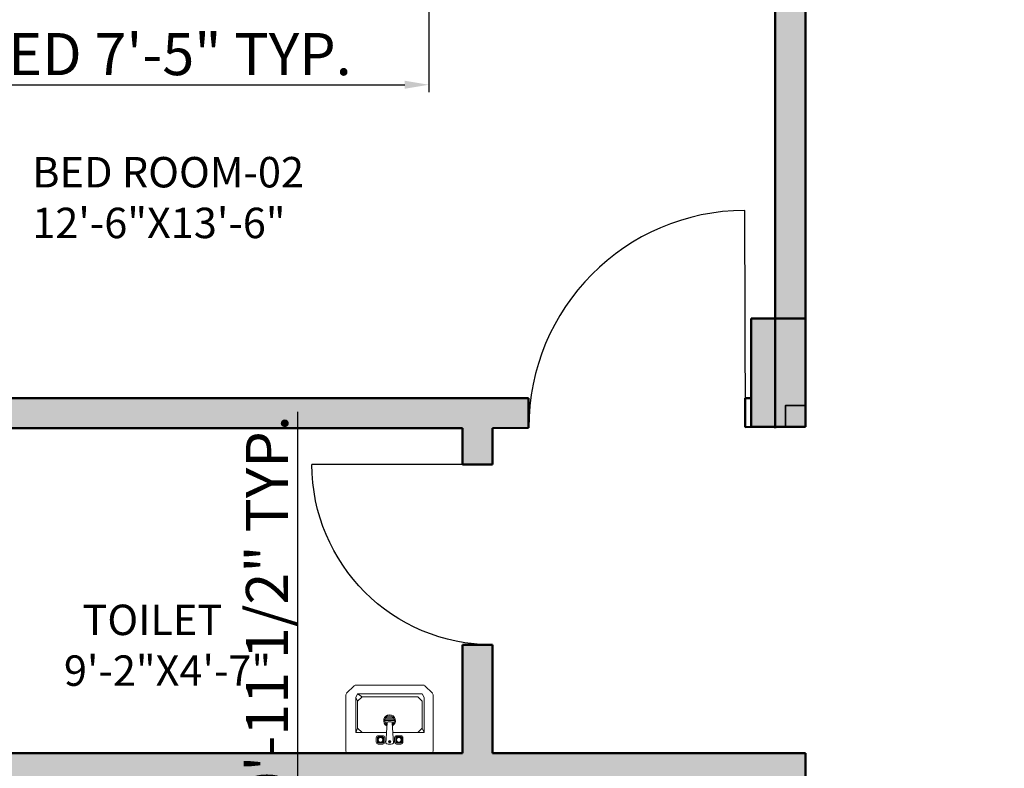
# Model space of a CAD drawing. Units: inches. Extents: x -7 to 1228, y -146 to 1091.
# Tile 10 of 88: x 105 to 269, y 276 to 401. Entities that reach past the tile are written whole.
import ezdxf

# ---------------------------------------------------------------- set-up
doc = ezdxf.new("R2010")
doc.units = ezdxf.units.IN
for name, color, linetype, lineweight in [('A-ANNO-DIMS', 2, 'Continuous', 18), ('A-AREA-IDEN', 7, 'Continuous', 18), ('A-COLS', 6, 'Continuous', 35), ('A-DOOR', 4, 'Continuous', 25), ('A-FURN', 8, 'Continuous', 18), ('A-WALL', 7, 'Continuous', 50), ('A-WALL-PATT', 251, 'Continuous', 13)]:
    doc.layers.add(name, color=color, linetype=linetype, lineweight=lineweight)
doc.styles.get("Standard").update_dxf_attribs({"font": 'arial.ttf'})
doc.dimstyles.new('ISO-25', dxfattribs={"dimtxt": 7, "dimasz": 4, "dimexe": 1.25, "dimexo": 0.625, "dimtad": 1, "dimdec": 1, "dimlunit": 3, "dimtxsty": 'Standard', "dimcen": 2.5, "dimadec": 0, "dimazin": 0, "dimtfac": 1, "dimtdec": 1, "dimtmove": 1, "dimatfit": 3, "dimfxl": 1, "dimarcsym": 0})

# ---------------------------------------------------------------- blocks, each defined once
blk = doc.blocks.new('A$C4CB854FF')
for p, q in [((0, 0.3675), (0, 0.0552)), ((0.4725, 0.38), (0.0125, 0.38)), ((0.1787, 0.329), (0.2034, 0.329)), ((0.2337, 0.329), (0.2502, 0.329)), ((0.3052, 0.329), (0.2804, 0.329)), ((0.485, 0.0552), (0.485, 0.3675)), ((0.1677, 0.2932), (0.1677, 0.318)), ((0.1745, 0.2919), (0.1745, 0.3194)), ((0.1773, 0.3221), (0.2048, 0.3221)), ((0.2048, 0.2891), (0.1773, 0.2891)), ((0.2034, 0.2822), (0.1787, 0.2822)), ((0.2075, 0.3194), (0.2075, 0.2919)), ((0.2144, 0.318), (0.2144, 0.2932)), ((0.2279, 0.2104), (0.2213, 0.3235)), ((0.2625, 0.3235), (0.256, 0.2104)), ((0.2694, 0.318), (0.2694, 0.2932)), ((0.2763, 0.3194), (0.2763, 0.2919)), ((0.3065, 0.3221), (0.279, 0.3221)), ((0.279, 0.2891), (0.3065, 0.2891)), ((0.2804, 0.2822), (0.3052, 0.2822)), ((0.3093, 0.2919), (0.3093, 0.3194)), ((0.3162, 0.2932), (0.3162, 0.318)), ((0.05, 0.265), (0.2247, 0.265)), ((0.06, 0.24), (0.05, 0.265)), ((0.05, 0.07), (0.05, 0.265)), ((0.085, 0.265), (0.06, 0.24)), ((0.06, 0.24), (0.06, 0.09)), ((0.2591, 0.265), (0.43, 0.265)), ((0.395, 0.265), (0.42, 0.24)), ((0.42, 0.24), (0.43, 0.265)), ((0.42, 0.24), (0.42, 0.09)), ((0.43, 0.07), (0.43, 0.265)), ((0.2152, 0.1984), (0.2694, 0.1984)), ((0.2297, 0.2066), (0.2165, 0.2066)), ((0.2681, 0.1901), (0.2165, 0.1901)), ((0.2272, 0.2149), (0.2208, 0.2149)), ((0.2638, 0.1819), (0.2208, 0.1819)), ((0.2533, 0.1736), (0.2313, 0.1736)), ((0.2505, 0.2052), (0.2334, 0.2052)), ((0.2681, 0.2066), (0.2541, 0.2066)), ((0.2638, 0.2149), (0.2566, 0.2149)), ((0.05, 0.07), (0.06, 0.05)), ((0.06, 0.09), (0.085, 0.065)), ((0.085, 0.065), (0.395, 0.065)), ((0.42, 0.09), (0.395, 0.065)), ((0.395, 0.065), (0.42, 0.05)), ((0.42, 0.09), (0.43, 0.07)), ((0.43, 0.07), (0.42, 0.05)), ((0.0037, 0.0463), (0.0463, 0.0037)), ((0.42, 0.05), (0.06, 0.05)), ((0.4387, 0.0037), (0.4813, 0.0463)), ((0.0552, 0), (0.4298, 0))]:
    blk.add_line(p, q)
for centre, radius in [((0.191, 0.3056), 0.0165), ((0.191, 0.3056), 0.0127), ((0.2419, 0.3152), 0.00688), ((0.2419, 0.3152), 0.00344), ((0.2928, 0.3056), 0.0165), ((0.2928, 0.3056), 0.0127)]:
    blk.add_circle(centre, radius)
for centre, radius, start, end in [((0.0125, 0.3675), 0.0125, 90, 180), ((0.1787, 0.318), 0.011, 90, 180), ((0.2034, 0.318), 0.011, 0, 90), ((0.2329, 0.314), 0.015, 87.1975, 140.7274), ((0.2509, 0.314), 0.015, 39.2726, 92.8025), ((0.2804, 0.318), 0.011, 90, 180), ((0.3052, 0.318), 0.011, 0, 90), ((0.4725, 0.3675), 0.0125, 0, 90), ((0.1787, 0.2932), 0.011, 180, 270), ((0.1773, 0.3194), 0.00275, 90, 180), ((0.1773, 0.2919), 0.00275, 180, 270), ((0.2034, 0.2932), 0.011, 270, 0), ((0.2048, 0.3194), 0.00275, 360, 90), ((0.2048, 0.2919), 0.00275, 270, 0), ((0.2804, 0.2932), 0.011, 180, 270), ((0.279, 0.3194), 0.00275, 90, 180), ((0.279, 0.2919), 0.00275, 180, 270), ((0.3052, 0.2932), 0.011, 270, 360), ((0.3065, 0.3194), 0.00275, 360, 90), ((0.3065, 0.2919), 0.00275, 270, 0), ((0.2423, 0.1984), 0.033, 118.6883, 62.8686), ((0.2423, 0.1984), 0.0271, 124.7758, 57.2247), ((0.2334, 0.2107), 0.0055, 183.3274, 270), ((0.2505, 0.2107), 0.0055, 270, 356.6726), ((0.0125, 0.0552), 0.0125, 180, 225), ((0.4725, 0.0552), 0.0125, 315, 0), ((0.0552, 0.0125), 0.0125, 225, 270), ((0.4298, 0.0125), 0.0125, 270, 315)]:
    blk.add_arc(centre, radius, start, end)
blk = doc.blocks.new('DOOR-750')
blk.add_line((30, 30), (30, 0))
blk.add_arc((30, 30), 30, 180, 270)
blk = doc.blocks.new('DOOR-900')
blk.add_line((36, 0), (36, 36))
blk.add_arc((36, 0), 36, 90, 180)
blk = doc.blocks.new('*D24')
at = {"layer": 'A-ANNO-DIMS', "color": 0, "lineweight": -2, "transparency": 16777216}
for p, q in [((84.44, 402.8), (84.44, 388.82)), ((173.43, 402.8), (173.43, 388.82)), ((88.44, 390.07), (169.43, 390.07))]:
    blk.add_line(p, q, dxfattribs=at)
at = {"layer": 'A-ANNO-DIMS', "color": 0, "transparency": 16777216}
for points in [[(88.44, 390.74), (88.44, 389.41), (84.44, 390.07)], [(169.43, 390.74), (169.43, 389.41), (173.43, 390.07)]]:
    blk.add_solid(points, dxfattribs=at)
at = {"layer": 'Defpoints', "color": 0, "transparency": 16777216}
for p in [(84.44, 403.42), (173.43, 403.42), (173.43, 390.07)]:
    blk.add_point(p, dxfattribs=at)
at = {"layer": 'A-ANNO-DIMS', "color": 0, "transparency": 16777216, "insert": (128.93, 394.26), "char_height": 7, "attachment_point": 5}
blk.add_mtext('BED 7\'-5" TYP.', dxfattribs=at)
blk = doc.blocks.new('*D32')
at = {"layer": 'A-ANNO-DIMS', "color": 0, "lineweight": -2, "transparency": 16777216}
for p, q in [((159.65, 262.03), (159.65, 259.24)), ((174.13, 262.03), (174.13, 259.24)), ((170.13, 260.49), (163.65, 260.49)), ((166.89, 260.49), (170.8, 247.44)), ((170.8, 247.44), (294.04, 247.44))]:
    blk.add_line(p, q, dxfattribs=at)
at = {"layer": 'A-ANNO-DIMS', "color": 0, "transparency": 16777216}
for points in [[(163.65, 261.15), (163.65, 259.82), (159.65, 260.49)], [(170.13, 261.15), (170.13, 259.82), (174.13, 260.49)]]:
    blk.add_solid(points, dxfattribs=at)
at = {"layer": 'Defpoints', "color": 0, "transparency": 16777216}
for p in [(159.65, 262.66), (174.13, 262.66), (159.65, 260.49)]:
    blk.add_point(p, dxfattribs=at)
at = {"layer": 'A-ANNO-DIMS', "color": 0, "transparency": 16777216, "insert": (232.42, 251.68), "char_height": 7, "attachment_point": 5}
blk.add_mtext('SINK / BASIN 1\'-2 1/2" TYP.', dxfattribs=at)
blk = doc.blocks.new('*D33')
at = {"layer": 'A-ANNO-DIMS', "color": 0, "lineweight": -2, "transparency": 16777216}
for p, q in [((151.67, 270.07), (151.67, 335.74)), ((159.03, 274), (156.23, 274)), ((157.48, 268.33), (151.67, 270.07)), ((157.48, 266.66), (157.48, 270)), ((159.03, 262.66), (156.23, 262.66))]:
    blk.add_line(p, q, dxfattribs=at)
at = {"layer": 'A-ANNO-DIMS', "color": 0, "transparency": 16777216}
for points in [[(156.81, 270), (158.15, 270), (157.48, 274)], [(156.81, 266.66), (158.15, 266.66), (157.48, 262.66)]]:
    blk.add_solid(points, dxfattribs=at)
at = {"layer": 'Defpoints', "color": 0, "transparency": 16777216}
for p in [(157.48, 274), (159.65, 274), (159.65, 262.66)]:
    blk.add_point(p, dxfattribs=at)
at = {"layer": 'A-ANNO-DIMS', "color": 0, "transparency": 16777216, "insert": (147.43, 302.9), "char_height": 7, "attachment_point": 5, "rotation": 90}
blk.add_mtext('0\'-11 1/2" TYP.', dxfattribs=at)

msp = doc.modelspace()

# ---------------------------------------------------------------- hatches: boundary and pattern name
at = {"layer": 'A-COLS'}
h = msp.add_hatch(color=256, dxfattribs=at)
h.dxf.hatch_style = 1
h.paths.add_polyline_path([(236, 351.24), (227, 351.24), (227, 333.24), (232.71, 333.24), (232.71, 336.78), (236, 336.78)])
h = msp.add_hatch(color=256, dxfattribs=at)
h.dxf.hatch_style = 1
h.paths.add_polyline_path([(232.71, 336.78), (232.71, 333.24), (236, 333.24), (236, 336.78)])
at = {"layer": 'A-WALL-PATT'}
h = msp.add_hatch(color=256, dxfattribs=at)
h.dxf.hatch_style = 1
h.paths.add_polyline_path([(69, 568), (60, 568), (60, 493), (63.29, 493), (69, 493)])
h.paths.add_polyline_path([(69, 662.41), (60, 662.41), (60, 586), (69, 586)], flags=17)
h.paths.add_polyline_path([(69, 723), (184, 723), (184, 734), (179, 734), (179, 728), (69, 728), (69, 741.62), (60, 741.62), (60, 698.41), (69, 698.41)], flags=17)
h.paths.add_polyline_path([(69, 782), (231, 782), (231, 728), (231, 723), (231, 586), (236, 586), (236, 787), (69, 787), (69, 800.13), (60, 800.13), (60, 765.62), (69, 765.62)])
h.paths.add_polyline_path([(184, 842), (189, 842), (189, 848), (173, 848), (173, 842), (179, 842), (179, 787), (184, 787)])
h.paths.add_polyline_path([(118.22, 69), (69, 69), (69, 60), (118.22, 60)])
h.paths.add_polyline_path([(227, 69), (154.22, 69), (154.22, 60), (227, 60)])
h.paths.add_polyline_path([(236, 60), (232.71, 60), (227, 60), (227, 36), (236, 36)])
h.paths.add_polyline_path([(389, 60), (380, 60), (380, 36), (389, 36)])
h.paths.add_polyline_path([(384, 181), (380, 181), (380, 115), (380, 78), (384, 78)])
h.paths.add_polyline_path([(380, 115), (334.55, 115), (334.55, 109), (380, 109)])
h.paths.add_polyline_path([(274.55, 115), (236, 115), (236, 201), (232.71, 201), (231, 201), (231, 78), (236, 78), (236, 109), (274.55, 109)])
h.paths.add_polyline_path([(69, 123), (60, 123), (60, 78), (69, 78)])
h.paths.add_polyline_path([(69, 201), (60, 201), (60, 159), (69, 159)])
h.paths.add_polyline_path([(143, 219), (69, 219), (69, 213), (143, 213)], flags=17)
h.paths.add_polyline_path([(189, 219), (184, 219), (184, 274), (231, 274), (231, 219), (236, 219), (236, 279), (184, 279), (184, 297), (179, 297), (179, 279), (69, 279), (69, 290.91), (60, 290.91), (60, 262.18), (69, 262.18), (69, 274), (179, 274), (179, 219), (173, 219), (173, 213), (189, 213)])
h.paths.add_polyline_path([(69, 238.18), (60, 238.18), (60, 219), (69, 219)], flags=17)
h.paths.add_polyline_path([(69, 333), (60, 333), (60, 314.91), (69, 314.91), (69, 316.96)])
h.paths.add_polyline_path([(190, 338), (184, 338), (69, 338), (69, 333), (179, 333), (179, 327), (184, 327), (184, 333.02), (190, 333.05)])
h.paths.add_polyline_path([(69, 386.81), (60, 386.81), (60, 351), (69, 351)])
h.paths.add_polyline_path([(69, 475), (60, 475), (60, 422.81), (69, 422.81)])
h.paths.add_polyline_path([(236, 475), (231, 475), (231, 351.24), (236, 351.24)])
h.paths.add_polyline_path([(384, 475), (380, 475), (380, 362), (384, 362)])
h.paths.add_polyline_path([(547, 307), (439, 307), (439, 356), (445, 356), (445, 362), (433, 362), (433, 307), (380, 307), (380, 244), (380, 241), (384, 241), (384, 301), (433, 301), (433, 277), (439, 277), (439, 301), (547, 301)])
h.paths.add_polyline_path([(547, 241), (439, 241), (439, 247), (433, 247), (433, 235), (547, 235)])
h.paths.add_polyline_path([(450, 69), (440.29, 69), (424.89, 69), (389, 69), (389, 60), (450, 60)])
h.paths.add_polyline_path([(547, 69), (486, 69), (486, 60), (547, 60)])
h.paths.add_polyline_path([(556, 148.27), (547, 148.27), (547, 78), (556, 78)])
h.paths.add_polyline_path([(556, 223), (547, 223), (547, 195), (547, 184.27), (556, 184.27)])
h.paths.add_polyline_path([(556, 311.19), (547, 311.19), (547, 273.08), (556, 273.08)])
h.paths.add_polyline_path([(556, 344), (552.71, 344), (547, 344), (547, 335.19), (556, 335.19)])
h.paths.add_polyline_path([(556, 249.08), (547, 249.08), (547, 241), (556, 241)])
h.paths.add_polyline_path([(547, 362), (475, 362), (475, 356), (547, 356)], flags=0)
h.paths.add_polyline_path([(556, 399.62), (547, 399.62), (547, 362), (556, 362)])
h.paths.add_polyline_path([(556, 475), (547, 475), (547, 435.62), (556, 435.62)])
h.paths.add_polyline_path([(547, 493), (389, 493), (389, 487), (547, 487)])
h.paths.add_polyline_path([(380, 493), (278, 493), (278, 487), (380, 487)])
h.paths.add_polyline_path([(227, 493), (69, 493), (69, 487), (227, 487)])
h.paths.add_polyline_path([(643, 122.44), (634, 122.44), (634, 78), (643, 78)])
h.paths.add_polyline_path([(702.5, 69), (692.79, 69), (677.39, 69), (643, 69), (643, 60), (702.5, 60)])
h.paths.add_polyline_path([(798, 69), (738.5, 69), (738.5, 60), (798, 60)])
h.paths.add_polyline_path([(807, 60), (803.71, 60), (798, 60), (798, 36), (807, 36)])
h.paths.add_polyline_path([(807, 109), (846.75, 109), (846.75, 115), (807, 115), (807, 159), (802, 159), (802, 78), (807, 78)])
h.paths.add_polyline_path([(807, 201), (802, 201), (802, 195), (807, 195)])
h.paths.add_polyline_path([(643, 201), (634, 201), (634, 158.44), (643, 158.44)])
h.paths.add_polyline_path([(756, 225), (751, 225), (751, 219), (643, 219), (643, 213), (756, 213)])
h.paths.add_polyline_path([(643, 240.85), (634, 240.85), (634, 219), (643, 219)])
h.paths.add_polyline_path([(643, 274), (643, 288.63), (634, 288.63), (634, 264.85), (643, 264.85)])
h.paths.add_polyline_path([(802, 279), (756, 279), (756, 297), (751, 297), (751, 279), (643, 279), (643, 274), (751, 274), (751, 255), (756, 255), (756, 274), (802, 274)])
h.paths.add_polyline_path([(807, 333), (803.71, 333), (802, 333), (802, 279), (802, 274), (802, 219), (807, 219)])
h.paths.add_polyline_path([(956, 182), (951, 182), (951, 115), (906.75, 115), (906.75, 109), (951, 109), (951, 78), (956, 78)])
h.paths.add_polyline_path([(960, 60), (951, 60), (951, 36), (960, 36)])
h.paths.add_polyline_path([(1021, 69), (1005.78, 69), (960, 69), (960, 60), (1021, 60)])
h.paths.add_polyline_path([(956, 224), (951, 224), (951, 218), (956, 218)])
h.paths.add_polyline_path([(956, 302), (1004, 302), (1004, 278), (1010, 278), (1010, 302), (1118, 302), (1118, 290.81), (1127, 290.81), (1127, 326.97), (1118, 326.97), (1118, 320.97), (1118, 307), (1010, 307), (1010, 356), (1016, 356), (1016, 362), (1004, 362), (1004, 307), (951, 307), (951, 244), (951, 242), (954.29, 242), (956, 242)])
h.paths.add_polyline_path([(643, 333), (634, 333), (634, 312.63), (643, 312.63), (643, 316.96)])
h.paths.add_polyline_path([(756, 338), (643, 338), (643, 333), (751, 333), (751, 327), (756, 327)])
h.paths.add_polyline_path([(643, 388), (634, 388), (634, 351), (643, 351)])
h.paths.add_polyline_path([(807, 357), (802, 357), (802, 351), (807, 351)])
h.paths.add_polyline_path([(807, 475), (802, 475), (802, 393), (807, 393)])
h.paths.add_polyline_path([(643, 475), (634, 475), (634, 424), (643, 424)])
h.paths.add_polyline_path([(798, 493), (643, 493), (643, 487), (798, 487)])
h.paths.add_polyline_path([(634, 493), (556, 493), (556, 487), (634, 487)])
h.paths.add_polyline_path([(813, 493), (807, 493), (807, 487), (813, 487)])
h.paths.add_polyline_path([(951, 493), (849, 493), (849, 487), (951, 487)])
h.paths.add_polyline_path([(956, 484), (951, 484), (951, 374), (956, 374)])
h.paths.add_polyline_path([(1109, 493), (969, 493), (969, 487), (1109, 487)])
h.paths.add_polyline_path([(1127, 484), (1118, 484), (1118, 450.64), (1127, 450.64)])
h.paths.add_polyline_path([(1127, 414.64), (1118, 414.64), (1118, 365), (1127, 365)])
h.paths.add_polyline_path([(1109, 362), (1046, 362), (1046, 356), (1109, 356)], flags=17)
h.paths.add_polyline_path([(1127, 356), (1123.45, 356), (1118, 356), (1118, 350.97), (1127, 350.97)], flags=0)
h.paths.add_polyline_path([(1127, 266.81), (1118, 266.81), (1118, 262.36), (1118, 242), (1127, 242)], flags=17)
h.paths.add_polyline_path([(1118, 242), (1010, 242), (1010, 248), (1004, 248), (1004, 237), (1118, 237)])
h.paths.add_polyline_path([(1127, 224), (1118, 224), (1118, 170), (1127, 170)])
h.paths.add_polyline_path([(1127, 134), (1118, 134), (1118, 78), (1127, 78)])
h.paths.add_polyline_path([(1118, 69), (1057, 69), (1057, 60), (1118, 60)])
h.paths.add_polyline_path([(227, 571.55), (227, 574), (69, 574), (69, 568), (227, 568)])
h.paths.add_polyline_path([(380, 571.55), (380, 574), (278, 574), (278, 568), (380, 568)])
h.paths.add_polyline_path([(242, 574), (236, 574), (236, 568), (242, 568)])
h.paths.add_polyline_path([(547, 571.55), (547, 574), (389, 574), (389, 568), (547, 568)])
h.paths.add_polyline_path([(384, 733), (380, 733), (380, 586), (384, 586)])
h.paths.add_polyline_path([(556, 646), (634, 646), (634, 655), (547, 655), (547, 586), (556, 586)])
h.paths.add_polyline_path([(634, 574), (556, 574), (556, 568), (634, 568)])
h.paths.add_polyline_path([(643, 655), (634, 655), (634, 586), (643, 586)])
h.paths.add_polyline_path([(798, 574), (643, 574), (643, 568), (798, 568)])
h.paths.add_polyline_path([(643, 663.85), (634, 663.85), (634, 655), (643, 655)])
h.paths.add_polyline_path([(556, 676.97), (547, 676.97), (547, 655), (556, 655)])
h.paths.add_polyline_path([(556, 733), (547, 733), (547, 712.97), (556, 712.97)])
h.paths.add_polyline_path([(643, 710), (634, 710), (634, 699.85), (643, 699.85)])
h.paths.add_polyline_path([(807, 668), (802, 668), (802, 586), (807, 586)])
h.paths.add_polyline_path([(951, 574), (849, 574), (849, 568), (951, 568)])
h.paths.add_polyline_path([(956, 691), (951, 691), (951, 577), (956, 577)])
h.paths.add_polyline_path([(1109, 574), (969, 574), (969, 568), (1109, 568)])
h.paths.add_polyline_path([(1127, 643.4), (1118, 643.4), (1118, 577), (1127, 577)])
h.paths.add_polyline_path([(1127, 568), (1123.45, 568), (1118, 568), (1118, 493), (1127, 493)])
h.paths.add_polyline_path([(1127, 733), (1118, 733), (1118, 679.4), (1127, 679.4)])
h.paths.add_polyline_path([(1127, 777.35), (1118, 777.35), (1118, 770.04), (1118, 751), (1127, 751)], flags=17)
h.paths.add_polyline_path([(1118, 751), (1010, 751), (1010, 757), (1004, 757), (1004, 745), (1118, 745)])
h.paths.add_polyline_path([(956, 811), (1004, 811), (1004, 787), (1010, 787), (1010, 811), (1017.87, 811), (1017.87, 811.63, -0.414214), (1018.25, 812), (1031.98, 812, -0.414214), (1032.35, 811.63), (1032.35, 811), (1118, 811), (1118, 801.35), (1127, 801.35), (1127, 834.69), (1118, 834.69), (1118, 830.24), (1118, 817), (1010, 817), (1010, 866), (1016, 866), (1016, 872), (1004, 872), (1004, 817), (956, 817), (956, 866), (951, 866), (951, 751), (954.29, 751), (956, 751)])
h.paths.add_polyline_path([(1118, 872), (1046, 872), (1046, 866), (1118, 866)], flags=17)
h.paths.add_polyline_path([(1127, 924.71), (1118, 924.71), (1118, 884), (1127, 884)])
h.paths.add_polyline_path([(1127, 866), (1123.71, 866), (1118, 866), (1118, 858.69), (1127, 858.69)], flags=17)
h.paths.add_polyline_path([(956, 983), (951, 983), (951, 952), (807, 952), (807, 983), (802, 983), (802, 902), (807, 902), (807, 946), (951, 946), (951, 884), (956, 884)])
h.paths.add_polyline_path([(807, 842), (802, 842), (802, 787), (756, 787), (756, 806), (751, 806), (751, 787), (643, 787), (643, 782), (751, 782), (751, 764), (756, 764), (756, 782), (802, 782), (802, 728), (807, 728)])
h.paths.add_polyline_path([(756, 848), (643, 848), (643, 842), (751, 842), (751, 836), (756, 836)])
h.paths.add_polyline_path([(756, 734), (751, 734), (751, 728), (643, 728), (643, 723), (756, 723)])
h.paths.add_polyline_path([(643, 749.79), (634, 749.79), (634, 728), (637.29, 728), (643, 728)])
h.paths.add_polyline_path([(643, 805.41), (634, 805.41), (634, 773.79), (643, 773.79)])
h.paths.add_polyline_path([(643, 896.66), (634, 896.66), (634, 860), (637.29, 860), (643, 860)])
h.paths.add_polyline_path([(643, 842), (634, 842), (634, 829.41), (643, 829.41)])
h.paths.add_polyline_path([(643, 983), (634, 983), (634, 932.66), (643, 932.66)])
h.paths.add_polyline_path([(1127, 983), (1118, 983), (1118, 960.71), (1127, 960.71)])
h.paths.add_polyline_path([(1118, 1001), (1077.53, 1001), (1077.53, 992), (1118, 992)])
h.paths.add_polyline_path([(1041.53, 1001), (960, 1001), (960, 992), (1041.53, 992)])
h.paths.add_polyline_path([(960, 1025), (951, 1025), (951, 1001), (954.29, 1001), (960, 1001)])
h.paths.add_polyline_path([(807, 1025), (798, 1025), (798, 1001), (807, 1001)])
h.paths.add_polyline_path([(798, 1001), (738.5, 1001), (738.5, 992), (798, 992)])
h.paths.add_polyline_path([(702.5, 1001), (643, 1001), (643, 992), (702.5, 992)])
h.paths.add_polyline_path([(547, 1001), (499.11, 1001), (499.11, 992), (547, 992)])
h.paths.add_polyline_path([(463.11, 1001), (389, 1001), (389, 992), (463.11, 992)])
h.paths.add_polyline_path([(389, 1025), (380, 1025), (380, 1022), (380, 1001), (383.29, 1001), (389, 1001)])
h.paths.add_polyline_path([(236, 1025), (227, 1025), (227, 1001), (236, 1001)])
h.paths.add_polyline_path([(236, 983), (231, 983), (231, 860), (236, 860)])
h.paths.add_polyline_path([(274.55, 952), (236, 952), (236, 946), (274.55, 946)])
h.paths.add_polyline_path([(380, 952), (334.55, 952), (334.55, 946), (380, 946)])
h.paths.add_polyline_path([(384, 983), (380, 983), (380, 884), (383.29, 884), (384, 884)])
h.paths.add_polyline_path([(227, 1001), (155.01, 1001), (155.01, 992), (162.87, 992), (227, 992)])
h.paths.add_polyline_path([(119.01, 1001), (69, 1001), (69, 992), (119.01, 992)])
h.paths.add_polyline_path([(69, 983), (60, 983), (60, 922.99), (69, 922.99)])
h.paths.add_polyline_path([(69, 886.99), (60, 886.99), (60, 860), (63.29, 860), (69, 860)])
h.paths.add_polyline_path([(143, 848), (69, 848), (69, 842), (143, 842)])

# ---------------------------------------------------------------- linework, layer by layer
at = {"layer": 'A-COLS'}
msp.add_lwpolyline([(236, 333.24), (232.71, 333.24), (232.71, 336.78), (236, 336.78)], close=True, dxfattribs=at)
at = {"layer": 'A-WALL'}
for p, q in [((231, 493), (231, 333.22)), ((236, 493), (236, 333.24)), ((231, 338), (231, 487)), ((236, 333.24), (236, 487)), ((227, 333.24), (227, 351.24)), ((227, 351.24), (236, 351.24)), ((236, 351.24), (236, 333.24)), ((184, 338), (69, 338)), ((184, 338), (190, 338)), ((190, 333.05), (190, 338)), ((226, 333.2), (226, 338)), ((226, 338), (227, 338)), ((231, 338), (231, 333)), ((179, 333), (69, 333)), ((179, 327), (179, 333)), ((184, 333.02), (190, 333.05)), ((184, 327), (184, 333.02)), ((226, 333.2), (236, 333.24)), ((236, 333.24), (227, 333.24)), ((184, 327), (179, 327)), ((179, 279), (179, 297)), ((184, 297), (179, 297)), ((184, 279), (184, 297)), ((179, 279), (69, 279)), ((236, 279), (184, 279)), ((236, 274), (236, 279)), ((236, 279), (236, 115))]:
    msp.add_line(p, q, dxfattribs=at)

# ---------------------------------------------------------------- block references
at = {"layer": 'A-DOOR', "rotation": 0.1910794837966875}
msp.add_blockref('DOOR-900', (190.05, 333.07), dxfattribs=at)
at = {"layer": 'A-DOOR', "extrusion": (0, 0, -1), "zscale": -1, "rotation": 89.99999999999979}
msp.add_blockref('DOOR-750', (-154, 297), dxfattribs=at)
at = {"layer": 'A-FURN', "xscale": 29.84864686937646, "yscale": 29.84864686937646, "zscale": 29.84864686937646, "rotation": 180}
msp.add_blockref('A$C4CB854FF', (174.13, 290.34), dxfattribs=at)

# ---------------------------------------------------------------- texts
at = {"layer": 'A-AREA-IDEN', "char_height": 5.0568, "attachment_point": 1}
for s, insert in [('BED ROOM-02\\P12\'-6"X13\'-6"', (107.52, 378.07)), ('  TOILET\\P9\'-2"X4\'-7"', (112.78, 303.69))]:
    msp.add_mtext_dynamic_manual_height_columns(s, width=137.2821, gutter_width=25.28, heights=[0], dxfattribs=dict(at, insert=insert))

# ---------------------------------------------------------------- dimensions: what is measured, and where the dimension line sits
at = {"layer": 'A-ANNO-DIMS'}
dim = msp.add_linear_dim(base=(173.43, 390.07), p1=(84.44, 403.42), p2=(173.43, 403.42), text='BED <> TYP.', dimstyle='ISO-25', override={"dimdec": 1, "dimlfac": 1, "dimrnd": 0, "dimzin": 1, "dimdsep": 46, "dimlunit": 4, "dimfrac": 2}, dxfattribs=at)
dim.commit()
dim.dimension.update_dxf_attribs({"geometry": '*D24', "text_midpoint": (128.93, 394.26)})
for base, p1, p2, angle, text, picture, middle in [((157.48, 274), (159.65, 262.66), (159.65, 274), 90, '<> TYP.', '*D33', (147.43, 270.7)), ((159.65, 260.49), (174.13, 262.66), (159.65, 262.66), 180, 'SINK / BASIN <> TYP.', '*D32', (171.43, 251.68))]:
    dim = msp.add_linear_dim(base=base, p1=p1, p2=p2, angle=angle, text=text, dimstyle='ISO-25', override={"dimdec": 1, "dimlfac": 1, "dimrnd": 0, "dimzin": 1, "dimdsep": 46, "dimlunit": 4, "dimfrac": 2}, dxfattribs=at)
    dim.commit()
    dim.dimension.update_dxf_attribs({"geometry": picture, "text_midpoint": middle})

doc.saveas('drawing.dxf')
